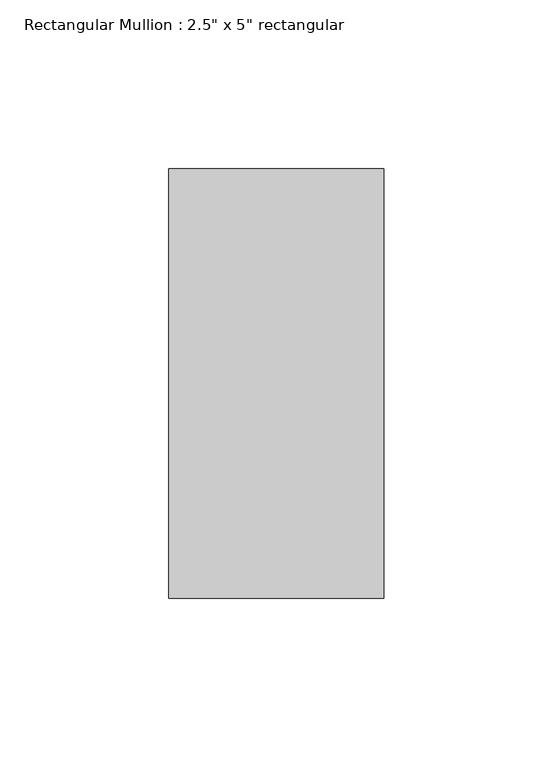
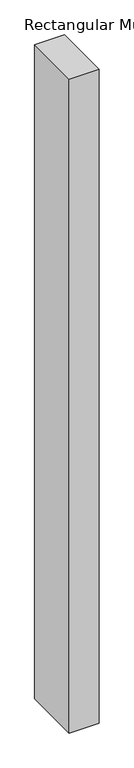
"""IFC4 building model written with IfcOpenShell, lengths in millimetres: member geometry."""

from ifc_helpers import new_model, si_unit, frame, origin, place, context, project, spatial, polyline, outline, extrude, source, transform, mapped, element, save


def member_a79ef8c7(model_context):
    return source(origin(), model_context, "Body", "SweptSolid", [
        extrude(outline(polyline([(0.0, 63.5), (0.0, -63.5), (-63.5, -63.5), (-63.5, 63.5), (0.0, 63.5)])), frame((0.0, 0.0, -1470.2926716), z_axis=(0.0, 0.0, 1.0), x_axis=(1.0, 0.0, 0.0)), (0.0, 0.0, 1.0), 1470.2926716),
    ])


if __name__ == "__main__":
    model = new_model("IFC4")
    model_context = context("Model", 3, world=origin())
    ifc_project = project(units=[si_unit("LENGTHUNIT", "METRE", prefix="MILLI")], contexts=[model_context])
    site = spatial("IfcSite", under=ifc_project)
    building = spatial("IfcBuilding", under=site)
    placement = place(None, origin())
    member_shape = member_a79ef8c7(model_context)
    element("IfcMember", 1, ObjectType="Rectangular Mullion : 2.5\" x 5\" rectangular", at=placement, inside=building, context=model_context, shape_type="MappedRepresentation", body=[
        mapped(member_shape, transform((0.0, 0.0, 0.0), x_axis=(1.0, 0.0, 0.0), y_axis=(0.0, 1.0, 0.0), z_axis=(0.0, 0.0, 1.0))),
    ])
    save(model, "model.ifc")

# Revit data of these elements
# Type "Rectangular Mullion : 2.5\" x 5\" rectangular"
#   built-in parameter 1007304 = 0.416667 (stored number, unit not read)
#   built-in parameter 1007301 = 0.104167 (stored number, unit not read)
#   built-in parameter 1007300 = 0.104167 (stored number, unit not read)
# Element 1 (IfcMember, "Rectangular Mullion : 2.5\" x 5\" rectangular")
#   Materials on its faces: "Aluminum"
# Materials
#   "Aluminum": class "Metal", colour RGB 247 247 247, transparency 0, Description = "Aluminum 6061", Cost = 0
